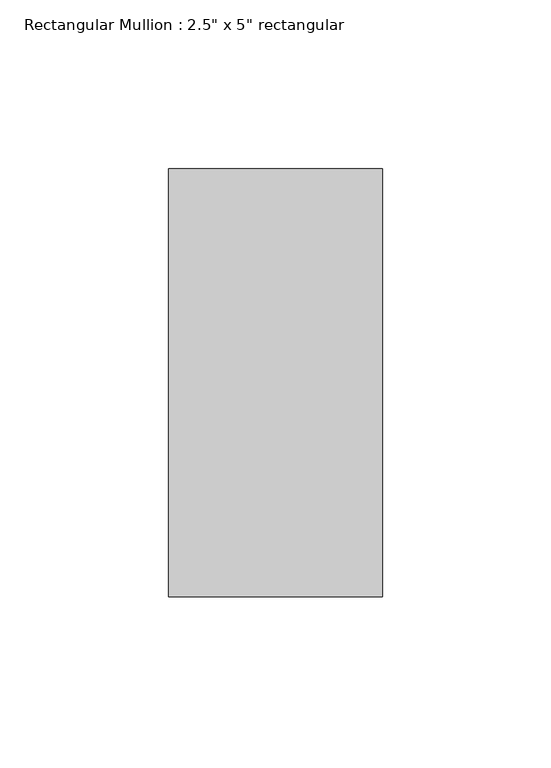
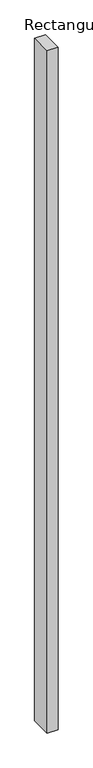
"""IFC4 building model written with IfcOpenShell, lengths in millimetres: member geometry."""

from ifc_helpers import new_model, si_unit, frame, origin, place, context, project, spatial, polyline, outline, extrude, source, transform, mapped, element, save


def member_6420ba3e(model_context):
    return source(origin(), model_context, "Body", "SweptSolid", [
        extrude(outline(polyline([(0.0, 63.5), (0.0, -63.5), (-63.5, -63.5), (-63.5, 63.5), (0.0, 63.5)])), frame((0.0, 0.0, -4230.04239), z_axis=(0.0, 0.0, 1.0), x_axis=(1.0, 0.0, 0.0)), (0.0, 0.0, 1.0), 4230.04239),
    ])


if __name__ == "__main__":
    model = new_model("IFC4")
    model_context = context("Model", 3, world=origin())
    ifc_project = project(units=[si_unit("LENGTHUNIT", "METRE", prefix="MILLI")], contexts=[model_context])
    site = spatial("IfcSite", under=ifc_project)
    building = spatial("IfcBuilding", under=site)
    placement = place(None, origin())
    member_shape = member_6420ba3e(model_context)
    element("IfcMember", 1, ObjectType="Rectangular Mullion : 2.5\" x 5\" rectangular", at=placement, inside=building, context=model_context, shape_type="MappedRepresentation", body=[
        mapped(member_shape, transform((0.0, 0.0, 0.0), x_axis=(1.0, 0.0, 0.0), y_axis=(0.0, 1.0, 0.0), z_axis=(0.0, 0.0, 1.0))),
    ])
    save(model, "model.ifc")

# Revit data of these elements
# Type "Rectangular Mullion : 2.5\" x 5\" rectangular"
#   built-in parameter 1007304 = 0.416667 (stored number, unit not read)
#   built-in parameter 1007301 = 0.104167 (stored number, unit not read)
#   built-in parameter 1007300 = 0.104167 (stored number, unit not read)
# Element 1 (IfcMember, "Rectangular Mullion : 2.5\" x 5\" rectangular")
#   Materials on its faces: "Aluminum"
# Materials
#   "Aluminum": class "Metal", colour RGB 247 247 247, transparency 0, Description = "Aluminum 6061", Cost = 0
